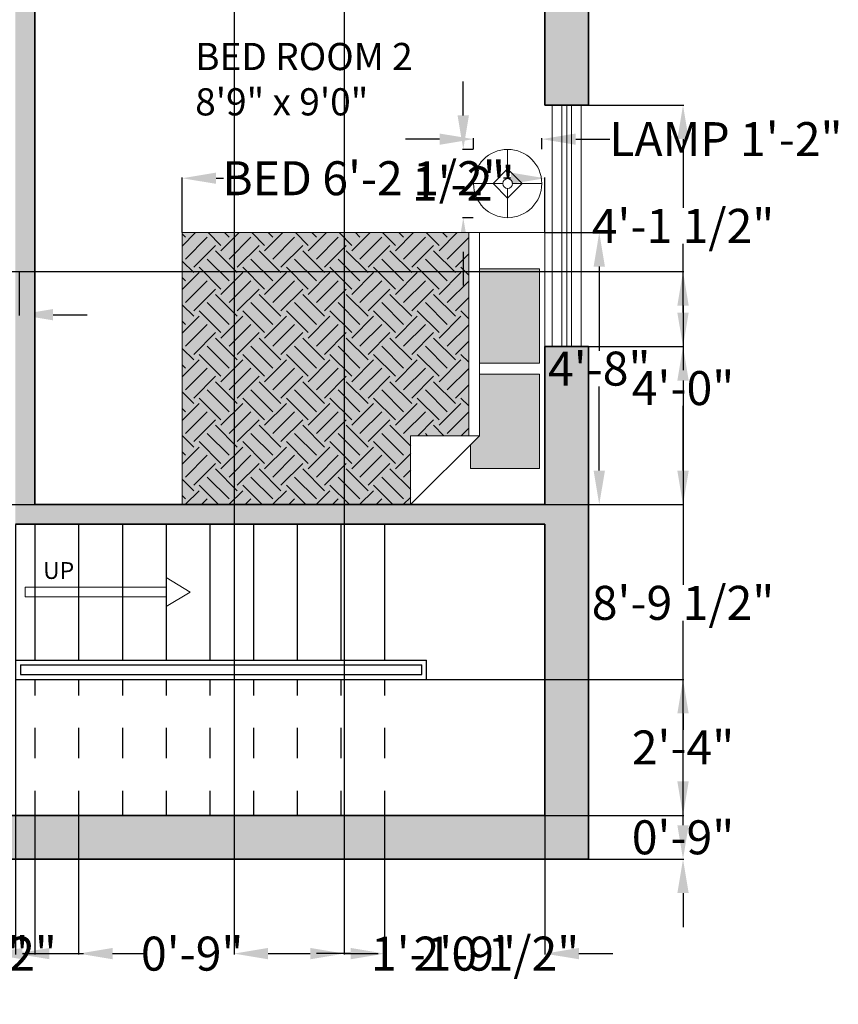
# Model space of a CAD drawing. Units: inches. Extents: x -8 to 329, y 10 to 430.
# Tile 2 of 4: x 153 to 321, y 10 to 213. Entities that reach past the tile are written whole.
import ezdxf

# ---------------------------------------------------------------- set-up
doc = ezdxf.new("R2010")
doc.units = ezdxf.units.IN
doc.header["$MEASUREMENT"] = 0
for name, color, linetype, lineweight in [('A-ANNO-DIMS', 2, 'Continuous', 18), ('A-ANNO-SYMB', 7, 'Continuous', 18), ('A-ANNO-TEXT', 7, 'Continuous', 18), ('A-AREA-IDEN', 7, 'Continuous', 18), ('A-FLOR-STRS', 7, 'Continuous', 25), ('A-FURN', 8, 'Continuous', 18), ('A-GLAZ', 4, 'Continuous', 18), ('A-WALL', 7, 'Continuous', 35), ('A-WALL-PATT', 253, 'Continuous', 13)]:
    doc.layers.add(name, color=color, linetype=linetype, lineweight=lineweight)
doc.layers.add('A-FURN-BASE-PATT', color=144, linetype='Continuous', lineweight=13, true_color=0x1e788f)
doc.layers.add('A-FURN-PATT', color=39, linetype='Continuous', lineweight=13, true_color=0x603913)
doc.styles.get("Standard").update_dxf_attribs({"font": 'arial.ttf'})
doc.dimstyles.get("Standard").update_dxf_attribs({"dimtxt": 7, "dimasz": 7, "dimexe": 0.18, "dimexo": 0.0625, "dimgap": 0.09, "dimtad": 0, "dimtih": 1, "dimtoh": 1, "dimdec": 0, "dimzin": 0, "dimdsep": 46, "dimlunit": 3, "dimtxsty": 'Standard', "dimcen": 0.09, "dimadec": 0, "dimazin": 0, "dimtfac": 1, "dimtdec": 0, "dimtofl": 0, "dimtmove": 0, "dimatfit": 3, "dimfxl": 1, "dimtolj": 1, "dimtzin": 0, "dimarcsym": 0})
pattern_1 = [(45, (0, 0), (0, 8.98026), [6.35, -6.35]), (45, (-1.684, 1.684), (0, 8.98026), [6.35, -6.35]), (45, (-3.3676, 3.3676), (0, 8.98026), [6.35, -6.35]), (135, (-3.3676, 4.49), (-8.98026, 0), [6.35, -6.35]), (135, (-1.684, 6.174), (-8.98026, 0), [6.35, -6.35]), (135, (0, 7.858), (-8.98026, 0), [6.35, -6.35])]

# ---------------------------------------------------------------- blocks, each defined once
blk = doc.blocks.new('Bed - Queen')
for p, q in [((0, -80.00003), (0, 0)), ((0, 0), (59.99999, 0)), ((59.99999, 0), (59.99999, -80.00003)), ((7.99999, -1.2), (28.79998, -1.2)), ((7.99999, -14.4), (7.99999, -1.2)), ((28.79998, -1.2), (28.79998, -14.4)), ((31.19999, -1.2), (51.99999, -1.2)), ((31.19999, -14.4), (31.19999, -1.2)), ((51.99999, -1.2), (51.99999, -16.4)), ((0, -14.4), (44.8, -14.4)), ((59.99999, -29.6), (44.8, -14.4)), ((44.8, -14.4), (44.8, -29.6)), ((44.8, -16.8), (0, -16.8)), ((51.99999, -16.4), (46.79936, -16.4)), ((44.8, -29.6), (59.99999, -29.6)), ((59.99999, -80.00003), (0, -80.00003))]:
    blk.add_line(p, q)
blk = doc.blocks.new('Lamp - Table')
for p, q in [((0, 7), (0, 1)), ((0, 3), (-3, 0)), ((3, 0), (0, 3)), ((-1, 0), (-7, 0)), ((-3, 0), (0, -3)), ((0, -3), (3, 0)), ((1, 0), (7, 0)), ((0, -1), (0, -7))]:
    blk.add_line(p, q)
for radius in [7, 1]:
    blk.add_circle((0, 0), radius)
blk = doc.blocks.new('STAIR-RISER-BEYOND')
for p, q in [((0, 28), (0, 24.68)), ((0, 18.05), (0, 11.78)), ((0, 5.06), (0, 0))]:
    blk.add_line(p, q)
blk = doc.blocks.new('*D20')
at = {"layer": 'A-ANNO-DIMS', "color": 0, "lineweight": -2, "transparency": 16777216}
for p, q in [((186.22, 168.83), (186.22, 180.15)), ((193.22, 179.97), (194.76, 179.97)), ((253.9, 179.97), (252.37, 179.97)), ((260.9, 168.83), (260.9, 180.15))]:
    blk.add_line(p, q, dxfattribs=at)
at = {"layer": 'A-ANNO-DIMS', "color": 0, "transparency": 16777216}
for points in [[(193.22, 181.14), (193.22, 178.81), (186.22, 179.97)], [(253.9, 181.14), (253.9, 178.81), (260.9, 179.97)]]:
    blk.add_solid(points, dxfattribs=at)
at = {"layer": 'Defpoints', "color": 0, "transparency": 16777216}
for p in [(260.9, 179.97), (186.22, 168.77), (260.9, 168.77)]:
    blk.add_point(p, dxfattribs=at)
at = {"layer": 'A-ANNO-DIMS', "color": 0, "transparency": 16777216, "insert": (223.56, 179.97), "char_height": 7, "attachment_point": 5}
blk.add_mtext('\\A1;BED 6\'-2 1/2"', dxfattribs=at)
blk = doc.blocks.new('*D21')
at = {"layer": 'A-ANNO-DIMS', "color": 0, "lineweight": -2, "transparency": 16777216}
for p, q in [((260.96, 168.77), (272.28, 168.77)), ((272.1, 161.77), (272.1, 144.43)), ((272.1, 119.76), (272.1, 137.1)), ((260.96, 112.76), (272.28, 112.76))]:
    blk.add_line(p, q, dxfattribs=at)
at = {"layer": 'A-ANNO-DIMS', "color": 0, "transparency": 16777216}
for points in [[(270.94, 161.77), (273.27, 161.77), (272.1, 168.77)], [(270.94, 119.76), (273.27, 119.76), (272.1, 112.76)]]:
    blk.add_solid(points, dxfattribs=at)
at = {"layer": 'Defpoints', "color": 0, "transparency": 16777216}
for p in [(260.9, 168.77), (260.9, 112.76), (272.1, 112.76)]:
    blk.add_point(p, dxfattribs=at)
at = {"layer": 'A-ANNO-DIMS', "color": 0, "transparency": 16777216, "insert": (272.1, 140.77), "char_height": 7, "attachment_point": 5}
blk.add_mtext('\\A1;4\'-8"', dxfattribs=at)
blk = doc.blocks.new('*D26')
at = {"layer": 'A-ANNO-DIMS', "color": 0, "lineweight": -2, "transparency": 16777216}
for p, q in [((239.21, 188.02), (232.21, 188.02)), ((246.21, 185.97), (246.21, 188.2)), ((260.27, 185.97), (260.27, 188.2)), ((267.27, 188.02), (274.27, 188.02))]:
    blk.add_line(p, q, dxfattribs=at)
at = {"layer": 'A-ANNO-DIMS', "color": 0, "transparency": 16777216}
for points in [[(239.21, 189.18), (239.21, 186.85), (246.21, 188.02)], [(267.27, 189.18), (267.27, 186.85), (260.27, 188.02)]]:
    blk.add_solid(points, dxfattribs=at)
at = {"layer": 'Defpoints', "color": 0, "transparency": 16777216}
for p in [(260.27, 188.02), (246.21, 185.91), (260.27, 185.91)]:
    blk.add_point(p, dxfattribs=at)
at = {"layer": 'A-ANNO-DIMS', "color": 0, "transparency": 16777216, "insert": (298.18, 188.02), "char_height": 7, "attachment_point": 5}
blk.add_mtext('\\A1;LAMP 1\'-2"', dxfattribs=at)
blk = doc.blocks.new('*D27')
at = {"layer": 'A-ANNO-DIMS', "color": 0, "lineweight": -2, "transparency": 16777216}
for p, q in [((244.1, 192.91), (244.1, 199.91)), ((246.15, 185.91), (243.92, 185.91)), ((246.15, 171.85), (243.92, 171.85)), ((244.1, 164.85), (244.1, 157.85))]:
    blk.add_line(p, q, dxfattribs=at)
at = {"layer": 'A-ANNO-DIMS', "color": 0, "transparency": 16777216}
for points in [[(242.93, 192.91), (245.27, 192.91), (244.1, 185.91)], [(242.93, 164.85), (245.27, 164.85), (244.1, 171.85)]]:
    blk.add_solid(points, dxfattribs=at)
at = {"layer": 'Defpoints', "color": 0, "transparency": 16777216}
for p in [(244.1, 185.91), (246.21, 185.91), (246.21, 171.85)]:
    blk.add_point(p, dxfattribs=at)
at = {"layer": 'A-ANNO-DIMS', "color": 0, "transparency": 16777216, "insert": (244.1, 178.88), "char_height": 7, "attachment_point": 5}
blk.add_mtext('\\A1;1\'-2"', dxfattribs=at)
blk = doc.blocks.new('*D33')
at = {"layer": 'A-ANNO-DIMS', "color": 0, "lineweight": -2, "transparency": 16777216}
for p, q in [((126.81, 160.68), (126.81, 151.69)), ((152.63, 160.68), (152.63, 151.69)), ((119.81, 151.87), (112.81, 151.87)), ((159.63, 151.87), (166.63, 151.87))]:
    blk.add_line(p, q, dxfattribs=at)
at = {"layer": 'A-ANNO-DIMS', "color": 0, "transparency": 16777216}
for points in [[(119.81, 153.04), (119.81, 150.71), (126.81, 151.87)], [(159.63, 153.04), (159.63, 150.71), (152.63, 151.87)]]:
    blk.add_solid(points, dxfattribs=at)
at = {"layer": 'Defpoints', "color": 0, "transparency": 16777216}
for p in [(126.81, 160.75), (152.63, 160.75), (152.63, 151.87)]:
    blk.add_point(p, dxfattribs=at)
at = {"layer": 'A-ANNO-DIMS', "color": 0, "transparency": 16777216, "insert": (139.72, 151.87), "char_height": 7, "attachment_point": 5}
blk.add_mtext('\\A1;2\'-2"', dxfattribs=at)
blk = doc.blocks.new('*D44')
at = {"layer": 'A-ANNO-DIMS', "color": 0, "lineweight": -2, "transparency": 16777216}
for p, q in [((122.79, 108.7), (122.79, 20.13)), ((151.9, 108.7), (151.9, 20.13)), ((115.79, 20.31), (108.79, 20.31)), ((158.9, 20.31), (165.9, 20.31))]:
    blk.add_line(p, q, dxfattribs=at)
at = {"layer": 'A-ANNO-DIMS', "color": 0, "transparency": 16777216}
for points in [[(115.79, 21.48), (115.79, 19.15), (122.79, 20.31)], [(158.9, 21.48), (158.9, 19.15), (151.9, 20.31)]]:
    blk.add_solid(points, dxfattribs=at)
at = {"layer": 'Defpoints', "color": 0, "transparency": 16777216}
for p in [(122.79, 108.76), (151.9, 108.76), (151.9, 20.31)]:
    blk.add_point(p, dxfattribs=at)
at = {"layer": 'A-ANNO-DIMS', "color": 0, "transparency": 16777216, "insert": (137.34, 20.31), "char_height": 7, "attachment_point": 5}
blk.add_mtext('\\A1;2\'-5"', dxfattribs=at)
blk = doc.blocks.new('*D48')
at = {"layer": 'A-ANNO-DIMS', "color": 0, "lineweight": -2, "transparency": 16777216}
for p, q in [((196.9, 226.25), (196.9, 20.13)), ((219.6, 226.7), (219.6, 20.13)), ((203.9, 20.31), (212.6, 20.31)), ((219.6, 20.31), (226.6, 20.31))]:
    blk.add_line(p, q, dxfattribs=at)
at = {"layer": 'A-ANNO-DIMS', "color": 0, "transparency": 16777216}
for points in [[(203.9, 21.48), (203.9, 19.15), (196.9, 20.31)], [(212.6, 21.48), (212.6, 19.15), (219.6, 20.31)]]:
    blk.add_solid(points, dxfattribs=at)
at = {"layer": 'Defpoints', "color": 0, "transparency": 16777216}
for p in [(196.9, 226.31), (219.6, 226.76), (219.6, 20.31)]:
    blk.add_point(p, dxfattribs=at)
at = {"layer": 'A-ANNO-DIMS', "color": 0, "transparency": 16777216, "insert": (246.54, 20.31), "char_height": 7, "attachment_point": 5}
blk.add_mtext('\\A1;1\'-10 1/2"', dxfattribs=at)
blk = doc.blocks.new('*D51')
at = {"layer": 'A-ANNO-DIMS', "color": 0, "lineweight": -2, "transparency": 16777216}
for p, q in [((98.9, 48.7), (98.9, 20.13)), ((87.54, 39.7), (87.54, 20.13)), ((80.54, 20.31), (73.54, 20.31)), ((105.9, 20.31), (112.9, 20.31))]:
    blk.add_line(p, q, dxfattribs=at)
at = {"layer": 'A-ANNO-DIMS', "color": 0, "transparency": 16777216}
for points in [[(80.54, 21.48), (80.54, 19.15), (87.54, 20.31)], [(105.9, 21.48), (105.9, 19.15), (98.9, 20.31)]]:
    blk.add_solid(points, dxfattribs=at)
at = {"layer": 'Defpoints', "color": 0, "transparency": 16777216}
for p in [(98.9, 48.76), (87.54, 39.76), (98.9, 20.31)]:
    blk.add_point(p, dxfattribs=at)
at = {"layer": 'A-ANNO-DIMS', "color": 0, "transparency": 16777216, "insert": (133.17, 20.31), "char_height": 7, "attachment_point": 5}
blk.add_mtext('\\A1;0\'-11 1/2"', dxfattribs=at)
blk = doc.blocks.new('*D57')
at = {"layer": 'A-ANNO-DIMS', "color": 0, "lineweight": -2, "transparency": 16777216}
for p, q in [((269.96, 195.02), (289.53, 195.02)), ((289.35, 188.02), (289.35, 173.87)), ((289.35, 152.31), (289.35, 166.45)), ((269.96, 145.31), (289.53, 145.31))]:
    blk.add_line(p, q, dxfattribs=at)
at = {"layer": 'A-ANNO-DIMS', "color": 0, "transparency": 16777216}
for points in [[(288.18, 188.02), (290.52, 188.02), (289.35, 195.02)], [(288.18, 152.31), (290.52, 152.31), (289.35, 145.31)]]:
    blk.add_solid(points, dxfattribs=at)
at = {"layer": 'Defpoints', "color": 0, "transparency": 16777216}
for p in [(269.9, 195.02), (269.9, 145.31), (289.35, 145.31)]:
    blk.add_point(p, dxfattribs=at)
at = {"layer": 'A-ANNO-DIMS', "color": 0, "transparency": 16777216, "insert": (289.35, 170.16), "char_height": 7, "attachment_point": 5}
blk.add_mtext('\\A1;4\'-1 1/2"', dxfattribs=at)
blk = doc.blocks.new('*D64')
at = {"layer": 'A-ANNO-DIMS', "color": 0, "lineweight": -2, "transparency": 16777216}
for p, q in [((269.96, 145.31), (289.53, 145.31)), ((289.35, 138.31), (289.35, 96.24)), ((289.35, 46.76), (289.35, 88.83)), ((269.96, 39.76), (289.53, 39.76))]:
    blk.add_line(p, q, dxfattribs=at)
at = {"layer": 'A-ANNO-DIMS', "color": 0, "transparency": 16777216}
for points in [[(288.18, 138.31), (290.52, 138.31), (289.35, 145.31)], [(288.18, 46.76), (290.52, 46.76), (289.35, 39.76)]]:
    blk.add_solid(points, dxfattribs=at)
at = {"layer": 'Defpoints', "color": 0, "transparency": 16777216}
for p in [(269.9, 145.31), (289.35, 145.31), (269.9, 39.76)]:
    blk.add_point(p, dxfattribs=at)
at = {"layer": 'A-ANNO-DIMS', "color": 0, "transparency": 16777216, "insert": (289.35, 92.54), "char_height": 7, "attachment_point": 5}
blk.add_mtext('\\A1;8\'-9 1/2"', dxfattribs=at)
blk = doc.blocks.new('*D66')
at = {"layer": 'A-ANNO-DIMS', "color": 0, "lineweight": -2, "transparency": 16777216}
for p, q in [((155.9, 48.7), (155.9, 20.13)), ((164.9, 48.7), (164.9, 20.13)), ((148.9, 20.31), (141.9, 20.31)), ((171.9, 20.31), (178.9, 20.31))]:
    blk.add_line(p, q, dxfattribs=at)
at = {"layer": 'A-ANNO-DIMS', "color": 0, "transparency": 16777216}
for points in [[(148.9, 21.48), (148.9, 19.15), (155.9, 20.31)], [(171.9, 21.48), (171.9, 19.15), (164.9, 20.31)]]:
    blk.add_solid(points, dxfattribs=at)
at = {"layer": 'Defpoints', "color": 0, "transparency": 16777216}
for p in [(155.9, 48.76), (164.9, 48.76), (164.9, 20.31)]:
    blk.add_point(p, dxfattribs=at)
at = {"layer": 'A-ANNO-DIMS', "color": 0, "transparency": 16777216, "insert": (188.29, 20.31), "char_height": 7, "attachment_point": 5}
blk.add_mtext('\\A1;0\'-9"', dxfattribs=at)
blk = doc.blocks.new('*D67')
at = {"layer": 'A-ANNO-DIMS', "color": 0, "lineweight": -2, "transparency": 16777216}
for p, q in [((227.9, 48.7), (227.9, 20.13)), ((260.9, 48.7), (260.9, 20.13)), ((220.9, 20.31), (213.9, 20.31)), ((267.9, 20.31), (274.9, 20.31))]:
    blk.add_line(p, q, dxfattribs=at)
at = {"layer": 'A-ANNO-DIMS', "color": 0, "transparency": 16777216}
for points in [[(220.9, 21.48), (220.9, 19.15), (227.9, 20.31)], [(267.9, 21.48), (267.9, 19.15), (260.9, 20.31)]]:
    blk.add_solid(points, dxfattribs=at)
at = {"layer": 'Defpoints', "color": 0, "transparency": 16777216}
for p in [(227.9, 48.76), (260.9, 48.76), (260.9, 20.31)]:
    blk.add_point(p, dxfattribs=at)
at = {"layer": 'A-ANNO-DIMS', "color": 0, "transparency": 16777216, "insert": (244.4, 20.31), "char_height": 7, "attachment_point": 5}
blk.add_mtext('\\A1;2\'-9"', dxfattribs=at)
blk = doc.blocks.new('*D68')
at = {"layer": 'A-ANNO-DIMS', "color": 0, "lineweight": -2, "transparency": 16777216}
for p, q in [((227.96, 76.76), (289.53, 76.76)), ((289.35, 69.76), (289.35, 66.37)), ((289.35, 55.76), (289.35, 59.16)), ((227.96, 48.76), (289.53, 48.76))]:
    blk.add_line(p, q, dxfattribs=at)
at = {"layer": 'A-ANNO-DIMS', "color": 0, "transparency": 16777216}
for points in [[(288.18, 69.76), (290.52, 69.76), (289.35, 76.76)], [(288.18, 55.76), (290.52, 55.76), (289.35, 48.76)]]:
    blk.add_solid(points, dxfattribs=at)
at = {"layer": 'Defpoints', "color": 0, "transparency": 16777216}
for p in [(227.9, 76.76), (289.35, 76.76), (227.9, 48.76)]:
    blk.add_point(p, dxfattribs=at)
at = {"layer": 'A-ANNO-DIMS', "color": 0, "transparency": 16777216, "insert": (289.35, 62.76), "char_height": 7, "attachment_point": 5}
blk.add_mtext('\\A1;2\'-4"', dxfattribs=at)
blk = doc.blocks.new('*D69')
at = {"layer": 'A-ANNO-DIMS', "color": 0, "lineweight": -2, "transparency": 16777216}
for p, q in [((289.35, 55.76), (289.35, 62.76)), ((260.96, 48.76), (289.53, 48.76)), ((269.96, 39.76), (289.53, 39.76)), ((289.35, 32.76), (289.35, 25.76))]:
    blk.add_line(p, q, dxfattribs=at)
at = {"layer": 'A-ANNO-DIMS', "color": 0, "transparency": 16777216}
for points in [[(288.18, 55.76), (290.52, 55.76), (289.35, 48.76)], [(288.18, 32.76), (290.52, 32.76), (289.35, 39.76)]]:
    blk.add_solid(points, dxfattribs=at)
at = {"layer": 'Defpoints', "color": 0, "transparency": 16777216}
for p in [(260.9, 48.76), (289.35, 48.76), (269.9, 39.76)]:
    blk.add_point(p, dxfattribs=at)
at = {"layer": 'A-ANNO-DIMS', "color": 0, "transparency": 16777216, "insert": (289.35, 44.26), "char_height": 7, "attachment_point": 5}
blk.add_mtext('\\A1;0\'-9"', dxfattribs=at)
blk = doc.blocks.new('*D71')
at = {"layer": 'A-ANNO-DIMS', "color": 0, "lineweight": -2, "transparency": 16777216}
for p, q in [((102.9, 39.7), (102.9, 20.13)), ((146.32, 39.7), (146.32, 20.13)), ((95.9, 20.31), (88.9, 20.31)), ((153.32, 20.31), (160.32, 20.31))]:
    blk.add_line(p, q, dxfattribs=at)
at = {"layer": 'A-ANNO-DIMS', "color": 0, "transparency": 16777216}
for points in [[(95.9, 21.48), (95.9, 19.15), (102.9, 20.31)], [(153.32, 21.48), (153.32, 19.15), (146.32, 20.31)]]:
    blk.add_solid(points, dxfattribs=at)
at = {"layer": 'Defpoints', "color": 0, "transparency": 16777216}
for p in [(102.9, 39.76), (146.32, 39.76), (146.32, 20.31)]:
    blk.add_point(p, dxfattribs=at)
at = {"layer": 'A-ANNO-DIMS', "color": 0, "transparency": 16777216, "insert": (124.61, 20.31), "char_height": 7, "attachment_point": 5}
blk.add_mtext('\\A1;3\'-7 1/2"', dxfattribs=at)
blk = doc.blocks.new('*D72')
at = {"layer": 'A-ANNO-DIMS', "color": 0, "lineweight": -2, "transparency": 16777216}
for p, q in [((126.87, 160.75), (289.53, 160.75)), ((289.35, 153.75), (289.35, 140.42)), ((289.35, 119.76), (289.35, 133.09)), ((122.85, 112.76), (289.53, 112.76))]:
    blk.add_line(p, q, dxfattribs=at)
at = {"layer": 'A-ANNO-DIMS', "color": 0, "transparency": 16777216}
for points in [[(288.18, 153.75), (290.52, 153.75), (289.35, 160.75)], [(288.18, 119.76), (290.52, 119.76), (289.35, 112.76)]]:
    blk.add_solid(points, dxfattribs=at)
at = {"layer": 'Defpoints', "color": 0, "transparency": 16777216}
for p in [(126.81, 160.75), (122.79, 112.76), (289.35, 112.76)]:
    blk.add_point(p, dxfattribs=at)
at = {"layer": 'A-ANNO-DIMS', "color": 0, "transparency": 16777216, "insert": (289.35, 136.76), "char_height": 7, "attachment_point": 5}
blk.add_mtext('\\A1;4\'-0"', dxfattribs=at)
blk = doc.blocks.new('*D74')
at = {"layer": 'A-ANNO-DIMS', "color": 0, "lineweight": -2, "transparency": 16777216}
for p, q in [((112.95, 168.66), (112.95, 20.13)), ((126.81, 160.68), (126.81, 20.13)), ((105.95, 20.31), (98.95, 20.31)), ((133.81, 20.31), (140.81, 20.31))]:
    blk.add_line(p, q, dxfattribs=at)
at = {"layer": 'A-ANNO-DIMS', "color": 0, "transparency": 16777216}
for points in [[(105.95, 21.48), (105.95, 19.15), (112.95, 20.31)], [(133.81, 21.48), (133.81, 19.15), (126.81, 20.31)]]:
    blk.add_solid(points, dxfattribs=at)
at = {"layer": 'Defpoints', "color": 0, "transparency": 16777216}
for p in [(112.95, 168.72), (126.81, 160.75), (126.81, 20.31)]:
    blk.add_point(p, dxfattribs=at)
at = {"layer": 'A-ANNO-DIMS', "color": 0, "transparency": 16777216, "insert": (149.87, 20.31), "char_height": 7, "attachment_point": 5}
blk.add_mtext('\\A1;1\'-2"', dxfattribs=at)

msp = doc.modelspace()

# ---------------------------------------------------------------- hatches: boundary and pattern name
at = {"layer": 'A-FURN-BASE-PATT'}
h = msp.add_hatch(color=256, dxfattribs=at)
h.dxf.hatch_style = 1
h.paths.add_polyline_path([(233.27, 112.76), (233.27, 126.95), (245.22, 126.95), (245.22, 168.77), (186.22, 168.77), (186.22, 112.76)])
h = msp.add_hatch(color=256, dxfattribs=at)
h.dxf.hatch_style = 1
h.paths.add_polyline_path([(259.78, 161.3), (247.46, 161.3), (247.46, 141.89), (259.78, 141.89)])
h = msp.add_hatch(color=256, dxfattribs=at)
h.dxf.hatch_style = 1
h.paths.add_polyline_path([(259.78, 139.65), (247.46, 139.65), (247.46, 126.95), (245.59, 125.09), (245.59, 120.23), (259.78, 120.23)])
at = {"layer": 'A-FURN-PATT'}
h = msp.add_hatch(dxfattribs=at)
h.set_pattern_fill('EARTH', color=256, angle=45)
h.set_pattern_definition(pattern_1)
h.paths.add_polyline_path([(186.22, 112.76), (233.27, 112.76), (233.27, 126.95), (245.22, 126.95), (245.22, 168.77), (186.22, 168.77)])
h = msp.add_hatch(dxfattribs=at)
h.set_pattern_fill('EARTH', color=256, angle=45)
h.set_pattern_definition(pattern_1)
h.paths.add_polyline_path([(186.22, 168.77), (186.22, 112.76), (233.27, 112.76), (233.27, 126.95), (245.22, 126.95), (245.22, 168.77)])
at = {"layer": 'A-WALL-PATT'}
h = msp.add_hatch(color=256, dxfattribs=at)
h.dxf.hatch_style = 1
h.paths.add_polyline_path([(146.32, 48.76), (146.32, 39.76), (269.9, 39.76), (269.9, 145.31), (260.9, 145.31), (260.9, 112.76), (186.22, 112.76), (155.9, 112.76), (155.9, 222.76), (155.9, 239.44), (153.1, 239.44), (151.9, 239.44), (151.9, 222.76), (151.9, 108.76), (260.9, 108.76), (260.9, 48.76)])
h = msp.add_hatch(color=256, dxfattribs=at)
h.dxf.hatch_style = 1
h.paths.add_polyline_path([(269.9, 239.44), (262.4, 239.44), (262.4, 238.67), (260.9, 238.67), (260.9, 226.76), (219.6, 226.76), (219.6, 223.9), (219.6, 222.76), (260.9, 222.76), (260.9, 195.02), (269.9, 195.02)])

# ---------------------------------------------------------------- linework, layer by layer
at = {"layer": 'A-ANNO-SYMB'}
for p, q in [((182.9, 95.76), (182.9, 97.76)), ((182.9, 97.76), (187.87, 94.76)), ((153.9, 93.76), (153.9, 95.76)), ((153.9, 95.76), (155.9, 95.76)), ((155.9, 95.76), (182.9, 95.76)), ((155.9, 93.76), (153.9, 93.76)), ((155.9, 93.76), (182.9, 93.76)), ((155.9, 93.76), (155.9, 93.76)), ((182.9, 91.76), (187.87, 94.76)), ((182.9, 93.76), (182.9, 91.76))]:
    msp.add_line(p, q, dxfattribs=at)
at = {"layer": 'A-FLOR-STRS'}
for p, q in [((155.9, 108.76), (155.9, 80.76)), ((164.9, 108.76), (164.9, 80.76)), ((173.9, 108.76), (173.9, 80.76)), ((182.9, 108.76), (182.9, 80.76)), ((191.9, 108.76), (191.9, 80.76)), ((200.9, 108.76), (200.9, 80.76)), ((209.9, 108.76), (209.9, 80.76)), ((218.9, 108.76), (218.9, 80.76)), ((227.9, 108.76), (227.9, 80.76)), ((151.9, 80.76), (236.56, 80.76)), ((152.9, 79.76), (235.56, 79.76)), ((152.9, 79.76), (152.9, 77.76)), ((235.56, 77.76), (235.56, 79.76)), ((236.56, 76.76), (236.56, 80.76)), ((152.9, 77.76), (235.56, 77.76)), ((151.9, 76.76), (236.56, 76.76))]:
    msp.add_line(p, q, dxfattribs=at)
at = {"layer": 'A-GLAZ'}
for p, q in [((262.4, 195.02), (262.4, 145.31)), ((264.4, 195.02), (264.4, 145.31)), ((265.4, 195.02), (265.4, 145.31)), ((266.4, 195.02), (266.4, 145.31)), ((268.4, 195.02), (268.4, 145.31))]:
    msp.add_line(p, q, dxfattribs=at)
at = {"layer": 'A-WALL'}
for p, q in [((269.9, 239.44), (269.9, 195.02)), ((155.9, 222.76), (155.9, 112.76)), ((260.9, 222.76), (260.9, 195.02)), ((260.9, 195.02), (269.9, 195.02)), ((260.9, 145.31), (269.9, 145.31)), ((260.9, 145.31), (260.9, 112.76)), ((269.9, 145.31), (269.9, 39.76)), ((155.9, 112.76), (260.9, 112.76)), ((151.9, 108.76), (260.9, 108.76)), ((260.9, 108.76), (260.9, 48.76)), ((146.32, 48.76), (260.9, 48.76)), ((29.9, 39.76), (269.9, 39.76))]:
    msp.add_line(p, q, dxfattribs=at)

# ---------------------------------------------------------------- block references
at = {"layer": 'A-FLOR-STRS'}
for p in [(155.9, 48.76), (164.9, 48.76), (173.9, 48.76), (182.9, 48.76), (191.9, 48.76), (200.9, 48.76), (209.9, 48.76), (218.9, 48.76), (227.9, 48.76)]:
    msp.add_blockref('STAIR-RISER-BEYOND', p, dxfattribs=at)
at = {"layer": 'A-FURN', "xscale": 1.004284262790401, "yscale": 1.004284262790401, "zscale": 1.004284262790401}
msp.add_blockref('Lamp - Table', (253.24, 178.88), dxfattribs=at)
at = {"layer": 'A-FURN', "xscale": 0.9334601152547126, "yscale": 0.9334601152547126, "zscale": 0.9334601152547126, "rotation": 270}
msp.add_blockref('Bed - Queen', (260.9, 168.77), dxfattribs=at)

# ---------------------------------------------------------------- texts
at = {"layer": 'A-ANNO-TEXT', "insert": (157.59, 100.93), "char_height": 3.466, "attachment_point": 1}
msp.add_mtext_dynamic_manual_height_columns('UP', width=28.378, gutter_width=17.33, heights=[0], dxfattribs=at)
at = {"layer": 'A-AREA-IDEN', "insert": (188.9, 207.83), "char_height": 5.5954, "attachment_point": 1}
msp.add_mtext_dynamic_manual_height_columns('BED ROOM 2\\P8\'9" x 9\'0"', width=164.8422, gutter_width=27.98, heights=[0], dxfattribs=at)

# ---------------------------------------------------------------- dimensions: what is measured, and where the dimension line sits
at = {"layer": 'A-ANNO-DIMS'}
for base, p1, p2, picture, middle in [((219.6, 20.31), (196.9, 226.31), (219.6, 226.76), '*D48', (246.54, 20.31)), ((126.81, 20.31), (112.95, 168.72), (126.81, 160.75), '*D74', (149.87, 20.31)), ((152.63, 151.87), (126.81, 160.75), (152.63, 160.75), '*D33', (139.72, 151.87)), ((151.9, 20.31), (122.79, 108.76), (151.9, 108.76), '*D44', (137.34, 20.31)), ((98.9, 20.31), (87.54, 39.76), (98.9, 48.76), '*D51', (133.17, 20.31)), ((164.9, 20.31), (155.9, 48.76), (164.9, 48.76), '*D66', (188.29, 20.31)), ((260.9, 20.31), (227.9, 48.76), (260.9, 48.76), '*D67', (244.4, 20.31)), ((146.32, 20.31), (102.9, 39.76), (146.32, 39.76), '*D71', (124.61, 20.31))]:
    dim = msp.add_linear_dim(base=base, p1=p1, p2=p2, dimstyle='Standard', override={"dimdec": 1, "dimlfac": 1, "dimrnd": 0, "dimzin": 1, "dimdsep": 46, "dimlunit": 4, "dimfrac": 2}, dxfattribs=at)
    dim.commit()
    dim.dimension.update_dxf_attribs({"geometry": picture, "text_midpoint": middle})
for base, p1, p2, angle, picture, middle in [((244.1, 185.91), (246.21, 171.85), (246.21, 185.91), 90, '*D27', (244.1, 178.88)), ((289.35, 145.31), (269.9, 195.02), (269.9, 145.31), 90, '*D57', (289.35, 170.16)), ((272.1, 112.76), (260.9, 168.77), (260.9, 112.76), 270, '*D21', (272.1, 140.77)), ((289.35, 112.76), (126.81, 160.75), (122.79, 112.76), 90, '*D72', (289.35, 136.76)), ((289.3506, 145.3073), (269.9006, 39.7634), (269.9006, 145.3073), 90, '*D64', (289.3506, 92.5354)), ((289.35, 76.76), (227.9, 48.76), (227.9, 76.76), 90, '*D68', (289.35, 62.76)), ((289.35, 48.76), (269.9, 39.76), (260.9, 48.76), 90, '*D69', (289.35, 44.26))]:
    dim = msp.add_linear_dim(base=base, p1=p1, p2=p2, angle=angle, dimstyle='Standard', override={"dimdec": 1, "dimlfac": 1, "dimrnd": 0, "dimzin": 1, "dimdsep": 46, "dimlunit": 4, "dimfrac": 2}, dxfattribs=at)
    dim.commit()
    dim.dimension.update_dxf_attribs({"geometry": picture, "text_midpoint": middle})
for base, p1, p2, text, picture, middle in [((260.27, 188.02), (246.21, 185.91), (260.27, 185.91), 'LAMP <>', '*D26', (298.18, 188.02)), ((260.9, 179.97), (186.22, 168.77), (260.9, 168.77), 'BED <>', '*D20', (223.56, 179.97))]:
    dim = msp.add_linear_dim(base=base, p1=p1, p2=p2, text=text, dimstyle='Standard', override={"dimdec": 1, "dimlfac": 1, "dimrnd": 0, "dimzin": 1, "dimdsep": 46, "dimlunit": 4, "dimfrac": 2}, dxfattribs=at)
    dim.commit()
    dim.dimension.update_dxf_attribs({"geometry": picture, "text_midpoint": middle})

doc.saveas('drawing.dxf')
